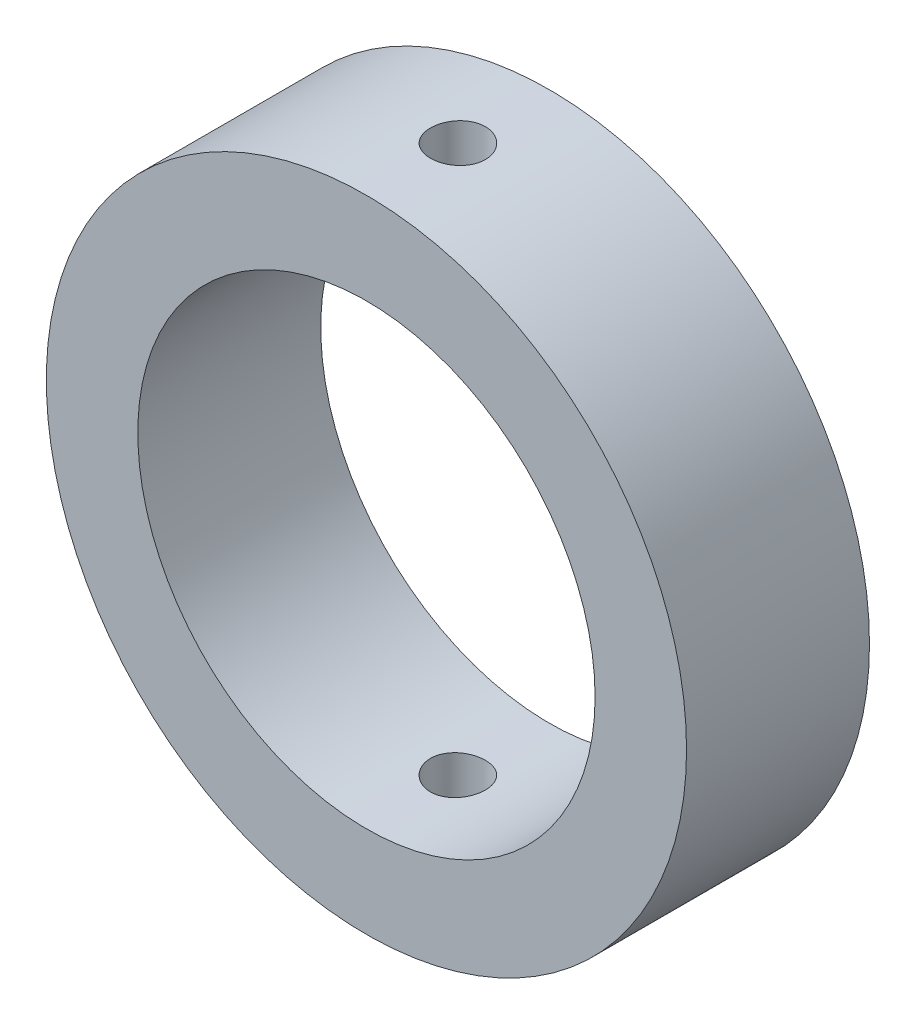
ISO-10303-21;
HEADER;
FILE_DESCRIPTION(('STEP AP214'),'2;1');
FILE_NAME('part.step','',(''),(''),'','','');
FILE_SCHEMA(('AUTOMOTIVE_DESIGN { 1 0 10303 214 1 1 1 1 }'));
ENDSEC;
DATA;
#1=APPLICATION_CONTEXT('core data for automotive mechanical design processes');
#2=APPLICATION_PROTOCOL_DEFINITION('international standard','automotive_design',2000,#1);
#3=PRODUCT_CONTEXT('',#1,'mechanical');
#4=PRODUCT('Part','Part','',(#3));
#5=PRODUCT_RELATED_PRODUCT_CATEGORY('part','',(#4));
#6=PRODUCT_DEFINITION_FORMATION('','',#4);
#7=PRODUCT_DEFINITION_CONTEXT('part definition',#1,'design');
#8=PRODUCT_DEFINITION('design','',#6,#7);
#9=PRODUCT_DEFINITION_SHAPE('','',#8);
#10=(LENGTH_UNIT() NAMED_UNIT(*) SI_UNIT(.MILLI.,.METRE.));
#11=(NAMED_UNIT(*) PLANE_ANGLE_UNIT() SI_UNIT($,.RADIAN.));
#12=(NAMED_UNIT(*) SI_UNIT($,.STERADIAN.) SOLID_ANGLE_UNIT());
#13=UNCERTAINTY_MEASURE_WITH_UNIT(LENGTH_MEASURE(1.E-05),#10,'distance_accuracy_value','');
#14=(GEOMETRIC_REPRESENTATION_CONTEXT(3) GLOBAL_UNCERTAINTY_ASSIGNED_CONTEXT((#13)) GLOBAL_UNIT_ASSIGNED_CONTEXT((#10,
#11,#12)) REPRESENTATION_CONTEXT('',''));
#15=CARTESIAN_POINT('',(0.,0.,0.));
#16=DIRECTION('',(0.,0.,1.));
#17=DIRECTION('',(1.,0.,0.));
#18=AXIS2_PLACEMENT_3D('',#15,#16,#17);
#19=CARTESIAN_POINT('',(0.,0.,20.));
#20=DIRECTION('',(0.,0.,1.));
#21=DIRECTION('',(1.,0.,0.));
#22=AXIS2_PLACEMENT_3D('',#19,#20,#21);
#23=PLANE('',#22);
#24=CARTESIAN_POINT('',(0.,0.,20.));
#25=DIRECTION('',(0.,0.,1.));
#26=DIRECTION('',(1.,0.,0.));
#27=AXIS2_PLACEMENT_3D('',#24,#25,#26);
#28=CIRCLE('',#27,35.);
#29=CARTESIAN_POINT('',(35.,0.,20.));
#30=VERTEX_POINT('',#29);
#31=EDGE_CURVE('E10',#30,#30,#28,.T.);
#32=ORIENTED_EDGE('',*,*,#31,.T.);
#33=EDGE_LOOP('',(#32));
#34=FACE_BOUND('',#33,.T.);
#35=CARTESIAN_POINT('',(0.,0.,20.));
#36=DIRECTION('',(0.,0.,1.));
#37=DIRECTION('',(1.,0.,0.));
#38=AXIS2_PLACEMENT_3D('',#35,#36,#37);
#39=CIRCLE('',#38,25.);
#40=CARTESIAN_POINT('',(25.,0.,20.));
#41=VERTEX_POINT('',#40);
#42=EDGE_CURVE('E57',#41,#41,#39,.T.);
#43=ORIENTED_EDGE('',*,*,#42,.F.);
#44=EDGE_LOOP('',(#43));
#45=FACE_BOUND('',#44,.T.);
#46=ADVANCED_FACE('F40',(#34,#45),#23,.T.);
#47=CARTESIAN_POINT('',(0.,0.,0.));
#48=DIRECTION('',(0.,0.,1.));
#49=DIRECTION('',(1.,0.,0.));
#50=AXIS2_PLACEMENT_3D('',#47,#48,#49);
#51=PLANE('',#50);
#52=CARTESIAN_POINT('',(0.,0.,0.));
#53=DIRECTION('',(0.,0.,1.));
#54=DIRECTION('',(1.,0.,0.));
#55=AXIS2_PLACEMENT_3D('',#52,#53,#54);
#56=CIRCLE('',#55,35.);
#57=CARTESIAN_POINT('',(35.,0.,0.));
#58=VERTEX_POINT('',#57);
#59=EDGE_CURVE('E51',#58,#58,#56,.T.);
#60=ORIENTED_EDGE('',*,*,#59,.F.);
#61=EDGE_LOOP('',(#60));
#62=FACE_BOUND('',#61,.T.);
#63=CARTESIAN_POINT('',(0.,0.,0.));
#64=DIRECTION('',(0.,0.,1.));
#65=DIRECTION('',(1.,0.,0.));
#66=AXIS2_PLACEMENT_3D('',#63,#64,#65);
#67=CIRCLE('',#66,25.);
#68=CARTESIAN_POINT('',(25.,0.,0.));
#69=VERTEX_POINT('',#68);
#70=EDGE_CURVE('E56',#69,#69,#67,.T.);
#71=ORIENTED_EDGE('',*,*,#70,.T.);
#72=EDGE_LOOP('',(#71));
#73=FACE_BOUND('',#72,.T.);
#74=ADVANCED_FACE('F92',(#62,#73),#51,.F.);
#75=CARTESIAN_POINT('',(0.,0.,20.));
#76=DIRECTION('',(0.,0.,-1.));
#77=DIRECTION('',(-1.,0.,0.));
#78=AXIS2_PLACEMENT_3D('',#75,#76,#77);
#79=CYLINDRICAL_SURFACE('',#78,35.);
#80=CARTESIAN_POINT('',(0.,-35.,13.));
#81=CARTESIAN_POINT('',(0.168180177421425,-34.9999983189466,12.9999926621086));
#82=CARTESIAN_POINT('',(0.336474410694065,-34.9987748870089,12.9858101377132));
#83=CARTESIAN_POINT('',(0.668405276387218,-34.9940120055983,12.9294427662291));
#84=CARTESIAN_POINT('',(0.832036433522409,-34.9904699418268,12.8872263096079));
#85=CARTESIAN_POINT('',(1.14978580604665,-34.9814700099417,12.7760219308489));
#86=CARTESIAN_POINT('',(1.30390939390644,-34.9760132356579,12.7070492915307));
#87=CARTESIAN_POINT('',(1.5983553572425,-34.9637955952331,12.5443180840418));
#88=CARTESIAN_POINT('',(1.7386806487592,-34.9570350055299,12.4505647683675));
#89=CARTESIAN_POINT('',(2.00196024172095,-34.9429478698077,12.2406617110507));
#90=CARTESIAN_POINT('',(2.12487233650439,-34.9356200130701,12.1244591132005));
#91=CARTESIAN_POINT('',(2.34947428548936,-34.9212352148941,11.8730679106441));
#92=CARTESIAN_POINT('',(2.45116320107853,-34.9141782854488,11.7378784666713));
#93=CARTESIAN_POINT('',(2.63057608789142,-34.9011203668809,11.4520942390574));
#94=CARTESIAN_POINT('',(2.70826279885841,-34.895121025662,11.3014759820008));
#95=CARTESIAN_POINT('',(2.83722803822898,-34.8848727505605,10.9892731041776));
#96=CARTESIAN_POINT('',(2.88850705745045,-34.8806237841455,10.8276886872931));
#97=CARTESIAN_POINT('',(2.96307845769353,-34.8743684880487,10.4985643557107));
#98=CARTESIAN_POINT('',(2.98643979537529,-34.8723566335604,10.3310401716124));
#99=CARTESIAN_POINT('',(3.00472573441206,-34.8707859372111,9.99443731566983));
#100=CARTESIAN_POINT('',(2.99965089755265,-34.8712270468893,9.82535867460139));
#101=CARTESIAN_POINT('',(2.96126551313284,-34.874507414771,9.49091935009246));
#102=CARTESIAN_POINT('',(2.92802995365881,-34.8773403039272,9.32554998866099));
#103=CARTESIAN_POINT('',(2.83438308452453,-34.8850750500347,9.00274549875546));
#104=CARTESIAN_POINT('',(2.77397149596722,-34.8899769282191,8.84531045172664));
#105=CARTESIAN_POINT('',(2.62760362876988,-34.9013046627491,8.5426048976093));
#106=CARTESIAN_POINT('',(2.54161375570937,-34.9077325210554,8.39735071245931));
#107=CARTESIAN_POINT('',(2.34655446417304,-34.9213861292491,8.12330862382476));
#108=CARTESIAN_POINT('',(2.23748455081154,-34.9286118962437,7.99452107351525));
#109=CARTESIAN_POINT('',(1.99894091774494,-34.9430754969892,7.75663207823613));
#110=CARTESIAN_POINT('',(1.86940237855328,-34.9503132942366,7.64759561833133));
#111=CARTESIAN_POINT('',(1.59382461581758,-34.9639632077666,7.45280656292255));
#112=CARTESIAN_POINT('',(1.44778538038973,-34.9703753234546,7.36705398418779));
#113=CARTESIAN_POINT('',(1.14330913680171,-34.9816527329005,7.2212707481009));
#114=CARTESIAN_POINT('',(0.984870717201058,-34.9865178502383,7.16124302414623));
#115=CARTESIAN_POINT('',(0.66011322112835,-34.9941511080319,7.06865924334512));
#116=CARTESIAN_POINT('',(0.493794317781497,-34.9969192945321,7.03610258328611));
#117=CARTESIAN_POINT('',(0.15856025083397,-35.0000408811527,6.99946669791016));
#118=CARTESIAN_POINT('',(-0.0103450366761302,-35.0004018916599,6.99529772286168));
#119=CARTESIAN_POINT('',(-0.346452104482659,-34.9986887867208,7.01532035576532));
#120=CARTESIAN_POINT('',(-0.513653901587615,-34.9966146953254,7.03951168360929));
#121=CARTESIAN_POINT('',(-0.841351421558966,-34.9902695086844,7.11549382233641));
#122=CARTESIAN_POINT('',(-1.00185687270474,-34.9860017297263,7.16724297716301));
#123=CARTESIAN_POINT('',(-1.31190702245475,-34.9757485102754,7.29682922006561));
#124=CARTESIAN_POINT('',(-1.46145153801856,-34.9697630411066,7.37466674367936));
#125=CARTESIAN_POINT('',(-1.7457428816744,-34.9567262474856,7.55444535294469));
#126=CARTESIAN_POINT('',(-1.88045202960912,-34.9496723123826,7.65644583152676));
#127=CARTESIAN_POINT('',(-2.13086824169311,-34.9352996751561,7.88156921992449));
#128=CARTESIAN_POINT('',(-2.24657495644839,-34.9279809681673,8.00469251803617));
#129=CARTESIAN_POINT('',(-2.45601016602155,-34.9138810732733,8.26895626973909));
#130=CARTESIAN_POINT('',(-2.54968004901865,-34.9071013498897,8.41014326356234));
#131=CARTESIAN_POINT('',(-2.71198063229128,-34.8948680127784,8.70629524502194));
#132=CARTESIAN_POINT('',(-2.78061159495576,-34.8894143851545,8.8612600882557));
#133=CARTESIAN_POINT('',(-2.8907865424564,-34.8804590783594,9.180362211124));
#134=CARTESIAN_POINT('',(-2.93236627395852,-34.8769548240937,9.34448707344406));
#135=CARTESIAN_POINT('',(-2.98737479633476,-34.872286503041,9.67742005737787));
#136=CARTESIAN_POINT('',(-3.0008041627162,-34.871122388412,9.84622808317732));
#137=CARTESIAN_POINT('',(-2.99912392353084,-34.8712668950776,10.1831530647903));
#138=CARTESIAN_POINT('',(-2.98410640669543,-34.8725675374248,10.3512704909289));
#139=CARTESIAN_POINT('',(-2.92615085557176,-34.8774780477604,10.6825859274482));
#140=CARTESIAN_POINT('',(-2.88321277999482,-34.8810879191635,10.8457839305537));
#141=CARTESIAN_POINT('',(-2.7706585792072,-34.8902080316544,11.1626330215739));
#142=CARTESIAN_POINT('',(-2.70104425727074,-34.8957181442861,11.3162847539864));
#143=CARTESIAN_POINT('',(-2.53712384137618,-34.9080181097009,11.6097355757974));
#144=CARTESIAN_POINT('',(-2.4428181018962,-34.9148079441114,11.7495348640265));
#145=CARTESIAN_POINT('',(-2.23184571903132,-34.9289284828144,12.0117838459397));
#146=CARTESIAN_POINT('',(-2.11511080731054,-34.9362607952504,12.1341785330169));
#147=CARTESIAN_POINT('',(-1.86271960746937,-34.9506254222313,12.357688026767));
#148=CARTESIAN_POINT('',(-1.72705875414518,-34.9576576638589,12.4587976843829));
#149=CARTESIAN_POINT('',(-1.44039065385252,-34.9706432183248,12.6370108284413));
#150=CARTESIAN_POINT('',(-1.28935405311577,-34.9765944046818,12.7140672103455));
#151=CARTESIAN_POINT('',(-0.976537475486436,-34.9867226680456,12.8416267776672));
#152=CARTESIAN_POINT('',(-0.814770058056751,-34.9909017781752,12.8921604088507));
#153=CARTESIAN_POINT('',(-0.543377751492647,-34.9959451685553,12.9524054943071));
#154=CARTESIAN_POINT('',(-0.4354969109927,-34.9974587860022,12.9702296244532));
#155=CARTESIAN_POINT('',(-0.218426750644092,-34.999486746251,12.9940292435666));
#156=CARTESIAN_POINT('',(-0.109237434508938,-35.0000010918883,13.0000047661528));
#157=CARTESIAN_POINT('',(0.,-35.,13.));
#158=B_SPLINE_CURVE_WITH_KNOTS('',3,(#80,#81,#82,#83,#84,#85,#86,#87,#88,#89,#90,#91,#92,#93,
#94,#95,#96,#97,#98,#99,#100,#101,#102,#103,#104,#105,#106,#107,#108,#109,#110,#111,#112,#113,
#114,#115,#116,#117,#118,#119,#120,#121,#122,#123,#124,#125,#126,#127,#128,#129,#130,#131,#132,
#133,#134,#135,#136,#137,#138,#139,#140,#141,#142,#143,#144,#145,#146,#147,#148,#149,#150,#151,
#152,#153,#154,#155,#156,#157),.UNSPECIFIED.,.T.,.F.,(4,2,2,2,2,2,2,2,2,2,2,2,2,2,2,2,2,2,2,2,2,
2,2,2,2,2,2,2,2,2,2,2,2,2,2,2,2,2,4),(0.,0.504141688620747,1.00885278730409,1.51327602436422,
2.01759242981481,2.5231110330061,3.0286519884333,3.53497383147415,4.04128626359052,
4.54634550220951,5.05139476290399,5.55510335902216,6.05881712462464,6.56319540924795,
7.06758450992202,7.57360414720597,8.07962414892789,8.58570183661505,9.09176841150507,
9.59623427417642,10.1006951543972,10.6043956535469,11.1081045622491,11.6130646830275,
12.1180340873686,12.6243317573245,13.1306241215114,13.636246082805,14.1418577070399,
14.6458353534655,15.1498137451707,15.6537580747011,16.1576951698375,16.6631911333163,
17.1688092410494,17.6754113983993,18.1814307424438,18.5088849156758,18.8363381597995),.UNSPECIFIED.);
#159=CARTESIAN_POINT('',(0.,-35.,13.));
#160=VERTEX_POINT('',#159);
#161=EDGE_CURVE('E84',#160,#160,#158,.T.);
#162=ORIENTED_EDGE('',*,*,#161,.T.);
#163=EDGE_LOOP('',(#162));
#164=FACE_BOUND('',#163,.T.);
#165=CARTESIAN_POINT('',(0.,35.,13.));
#166=CARTESIAN_POINT('',(-0.168180177421425,34.9999983189466,12.9999926621086));
#167=CARTESIAN_POINT('',(-0.336474410694065,34.9987748870089,12.9858101377132));
#168=CARTESIAN_POINT('',(-0.668405276387218,34.9940120055983,12.9294427662291));
#169=CARTESIAN_POINT('',(-0.832036433522409,34.9904699418268,12.8872263096079));
#170=CARTESIAN_POINT('',(-1.14978580604665,34.9814700099417,12.7760219308489));
#171=CARTESIAN_POINT('',(-1.30390939390644,34.9760132356579,12.7070492915307));
#172=CARTESIAN_POINT('',(-1.5983553572425,34.9637955952331,12.5443180840418));
#173=CARTESIAN_POINT('',(-1.7386806487592,34.9570350055299,12.4505647683675));
#174=CARTESIAN_POINT('',(-2.00196024172095,34.9429478698077,12.2406617110507));
#175=CARTESIAN_POINT('',(-2.12487233650439,34.9356200130701,12.1244591132005));
#176=CARTESIAN_POINT('',(-2.34947428548936,34.9212352148941,11.8730679106441));
#177=CARTESIAN_POINT('',(-2.45116320107853,34.9141782854488,11.7378784666713));
#178=CARTESIAN_POINT('',(-2.63057608789142,34.9011203668809,11.4520942390574));
#179=CARTESIAN_POINT('',(-2.70826279885841,34.895121025662,11.3014759820008));
#180=CARTESIAN_POINT('',(-2.83722803822898,34.8848727505605,10.9892731041776));
#181=CARTESIAN_POINT('',(-2.88850705745045,34.8806237841455,10.8276886872931));
#182=CARTESIAN_POINT('',(-2.96307845769353,34.8743684880487,10.4985643557107));
#183=CARTESIAN_POINT('',(-2.98643979537529,34.8723566335604,10.3310401716124));
#184=CARTESIAN_POINT('',(-3.00472573441206,34.8707859372111,9.99443731566983));
#185=CARTESIAN_POINT('',(-2.99965089755265,34.8712270468893,9.82535867460139));
#186=CARTESIAN_POINT('',(-2.96126551313284,34.874507414771,9.49091935009246));
#187=CARTESIAN_POINT('',(-2.92802995365881,34.8773403039272,9.32554998866099));
#188=CARTESIAN_POINT('',(-2.83438308452453,34.8850750500347,9.00274549875546));
#189=CARTESIAN_POINT('',(-2.77397149596722,34.8899769282191,8.84531045172664));
#190=CARTESIAN_POINT('',(-2.62760362876988,34.9013046627491,8.5426048976093));
#191=CARTESIAN_POINT('',(-2.54161375570937,34.9077325210554,8.39735071245931));
#192=CARTESIAN_POINT('',(-2.34655446417304,34.9213861292491,8.12330862382476));
#193=CARTESIAN_POINT('',(-2.23748455081154,34.9286118962437,7.99452107351525));
#194=CARTESIAN_POINT('',(-1.99894091774494,34.9430754969892,7.75663207823613));
#195=CARTESIAN_POINT('',(-1.86940237855328,34.9503132942366,7.64759561833133));
#196=CARTESIAN_POINT('',(-1.59382461581758,34.9639632077666,7.45280656292255));
#197=CARTESIAN_POINT('',(-1.44778538038973,34.9703753234546,7.36705398418779));
#198=CARTESIAN_POINT('',(-1.14330913680171,34.9816527329005,7.2212707481009));
#199=CARTESIAN_POINT('',(-0.984870717201058,34.9865178502383,7.16124302414623));
#200=CARTESIAN_POINT('',(-0.66011322112835,34.9941511080319,7.06865924334512));
#201=CARTESIAN_POINT('',(-0.493794317781497,34.9969192945321,7.03610258328611));
#202=CARTESIAN_POINT('',(-0.15856025083397,35.0000408811527,6.99946669791016));
#203=CARTESIAN_POINT('',(0.0103450366761302,35.0004018916599,6.99529772286168));
#204=CARTESIAN_POINT('',(0.346452104482659,34.9986887867208,7.01532035576532));
#205=CARTESIAN_POINT('',(0.513653901587615,34.9966146953254,7.03951168360929));
#206=CARTESIAN_POINT('',(0.841351421558966,34.9902695086844,7.11549382233641));
#207=CARTESIAN_POINT('',(1.00185687270474,34.9860017297263,7.16724297716301));
#208=CARTESIAN_POINT('',(1.31190702245475,34.9757485102754,7.29682922006561));
#209=CARTESIAN_POINT('',(1.46145153801856,34.9697630411066,7.37466674367936));
#210=CARTESIAN_POINT('',(1.7457428816744,34.9567262474856,7.55444535294469));
#211=CARTESIAN_POINT('',(1.88045202960912,34.9496723123826,7.65644583152676));
#212=CARTESIAN_POINT('',(2.13086824169311,34.9352996751561,7.88156921992449));
#213=CARTESIAN_POINT('',(2.24657495644839,34.9279809681673,8.00469251803617));
#214=CARTESIAN_POINT('',(2.45601016602155,34.9138810732733,8.26895626973909));
#215=CARTESIAN_POINT('',(2.54968004901865,34.9071013498897,8.41014326356234));
#216=CARTESIAN_POINT('',(2.71198063229128,34.8948680127784,8.70629524502194));
#217=CARTESIAN_POINT('',(2.78061159495576,34.8894143851545,8.8612600882557));
#218=CARTESIAN_POINT('',(2.8907865424564,34.8804590783594,9.180362211124));
#219=CARTESIAN_POINT('',(2.93236627395852,34.8769548240937,9.34448707344406));
#220=CARTESIAN_POINT('',(2.98737479633476,34.872286503041,9.67742005737787));
#221=CARTESIAN_POINT('',(3.0008041627162,34.871122388412,9.84622808317732));
#222=CARTESIAN_POINT('',(2.99912392353084,34.8712668950776,10.1831530647903));
#223=CARTESIAN_POINT('',(2.98410640669543,34.8725675374248,10.3512704909289));
#224=CARTESIAN_POINT('',(2.92615085557176,34.8774780477604,10.6825859274482));
#225=CARTESIAN_POINT('',(2.88321277999482,34.8810879191635,10.8457839305537));
#226=CARTESIAN_POINT('',(2.7706585792072,34.8902080316544,11.1626330215739));
#227=CARTESIAN_POINT('',(2.70104425727074,34.8957181442861,11.3162847539864));
#228=CARTESIAN_POINT('',(2.53712384137618,34.9080181097009,11.6097355757974));
#229=CARTESIAN_POINT('',(2.4428181018962,34.9148079441114,11.7495348640265));
#230=CARTESIAN_POINT('',(2.23184571903132,34.9289284828144,12.0117838459397));
#231=CARTESIAN_POINT('',(2.11511080731054,34.9362607952504,12.1341785330169));
#232=CARTESIAN_POINT('',(1.86271960746937,34.9506254222313,12.357688026767));
#233=CARTESIAN_POINT('',(1.72705875414518,34.9576576638589,12.4587976843829));
#234=CARTESIAN_POINT('',(1.44039065385252,34.9706432183248,12.6370108284413));
#235=CARTESIAN_POINT('',(1.28935405311577,34.9765944046818,12.7140672103455));
#236=CARTESIAN_POINT('',(0.976537475486436,34.9867226680456,12.8416267776672));
#237=CARTESIAN_POINT('',(0.814770058056751,34.9909017781752,12.8921604088507));
#238=CARTESIAN_POINT('',(0.543377751492647,34.9959451685553,12.9524054943071));
#239=CARTESIAN_POINT('',(0.4354969109927,34.9974587860022,12.9702296244532));
#240=CARTESIAN_POINT('',(0.218426750644092,34.999486746251,12.9940292435666));
#241=CARTESIAN_POINT('',(0.109237434508938,35.0000010918883,13.0000047661528));
#242=CARTESIAN_POINT('',(0.,35.,13.));
#243=B_SPLINE_CURVE_WITH_KNOTS('',3,(#165,#166,#167,#168,#169,#170,#171,#172,#173,#174,#175,
#176,#177,#178,#179,#180,#181,#182,#183,#184,#185,#186,#187,#188,#189,#190,#191,#192,#193,#194,
#195,#196,#197,#198,#199,#200,#201,#202,#203,#204,#205,#206,#207,#208,#209,#210,#211,#212,#213,
#214,#215,#216,#217,#218,#219,#220,#221,#222,#223,#224,#225,#226,#227,#228,#229,#230,#231,#232,
#233,#234,#235,#236,#237,#238,#239,#240,#241,#242),.UNSPECIFIED.,.T.,.F.,(4,2,2,2,2,2,2,2,2,2,2,
2,2,2,2,2,2,2,2,2,2,2,2,2,2,2,2,2,2,2,2,2,2,2,2,2,2,2,4),(0.,0.504141688620747,1.00885278730409,
1.51327602436422,2.01759242981481,2.5231110330061,3.0286519884333,3.53497383147415,
4.04128626359052,4.54634550220951,5.05139476290399,5.55510335902216,6.05881712462464,
6.56319540924795,7.06758450992202,7.57360414720597,8.07962414892789,8.58570183661505,
9.09176841150507,9.59623427417642,10.1006951543972,10.6043956535469,11.1081045622491,
11.6130646830275,12.1180340873686,12.6243317573245,13.1306241215114,13.636246082805,
14.1418577070399,14.6458353534655,15.1498137451707,15.6537580747011,16.1576951698375,
16.6631911333163,17.1688092410494,17.6754113983993,18.1814307424438,18.5088849156758,
18.8363381597995),.UNSPECIFIED.);
#244=CARTESIAN_POINT('',(0.,35.,13.));
#245=VERTEX_POINT('',#244);
#246=EDGE_CURVE('E76',#245,#245,#243,.T.);
#247=ORIENTED_EDGE('',*,*,#246,.T.);
#248=EDGE_LOOP('',(#247));
#249=FACE_BOUND('',#248,.T.);
#250=ORIENTED_EDGE('',*,*,#31,.F.);
#251=EDGE_LOOP('',(#250));
#252=FACE_BOUND('',#251,.T.);
#253=ORIENTED_EDGE('',*,*,#59,.T.);
#254=EDGE_LOOP('',(#253));
#255=FACE_BOUND('',#254,.T.);
#256=ADVANCED_FACE('F39',(#164,#249,#252,#255),#79,.T.);
#257=CARTESIAN_POINT('',(0.,0.,20.));
#258=DIRECTION('',(0.,0.,-1.));
#259=DIRECTION('',(-1.,0.,0.));
#260=AXIS2_PLACEMENT_3D('',#257,#258,#259);
#261=CYLINDRICAL_SURFACE('',#260,25.);
#262=CARTESIAN_POINT('',(0.,-25.,13.));
#263=CARTESIAN_POINT('',(0.167864047107699,-24.9999977357459,12.9999928360586));
#264=CARTESIAN_POINT('',(0.335834317331191,-24.9982914200408,12.9858633413073));
#265=CARTESIAN_POINT('',(0.66710457130825,-24.991648705422,12.9297189358446));
#266=CARTESIAN_POINT('',(0.830399429590069,-24.9867088933728,12.8876745587494));
#267=CARTESIAN_POINT('',(1.14747479534053,-24.9741559265426,12.776953723474));
#268=CARTESIAN_POINT('',(1.30126148759225,-24.9665445315309,12.7082947931758));
#269=CARTESIAN_POINT('',(1.595099157832,-24.9494959264345,12.5463312649167));
#270=CARTESIAN_POINT('',(1.73515256713516,-24.9400590404141,12.4530310402467));
#271=CARTESIAN_POINT('',(1.99829131534451,-24.920360105442,12.2439251380248));
#272=CARTESIAN_POINT('',(2.1212966913072,-24.9100945030904,12.1280191598881));
#273=CARTESIAN_POINT('',(2.34615931038342,-24.8899239397152,11.8772070351121));
#274=CARTESIAN_POINT('',(2.44801549826474,-24.8800189967068,11.7422999409814));
#275=CARTESIAN_POINT('',(2.62798342873896,-24.8616560370405,11.4567991747016));
#276=CARTESIAN_POINT('',(2.7060207567257,-24.8532025903971,11.3061582754199));
#277=CARTESIAN_POINT('',(2.8356605730156,-24.8387461344686,10.9937912978913));
#278=CARTESIAN_POINT('',(2.88726398696776,-24.8327430393798,10.8320656080307));
#279=CARTESIAN_POINT('',(2.96232930045399,-24.8239006073737,10.5029471406886));
#280=CARTESIAN_POINT('',(2.98592577987646,-24.8210461452543,10.3355854715723));
#281=CARTESIAN_POINT('',(3.0047237521967,-24.8187777690611,9.99925506363583));
#282=CARTESIAN_POINT('',(2.99992630052848,-24.8193637271033,9.83028638478303));
#283=CARTESIAN_POINT('',(2.96218316078668,-24.8238961466306,9.49647403521565));
#284=CARTESIAN_POINT('',(2.92938543222303,-24.8278249434675,9.33161336131982));
#285=CARTESIAN_POINT('',(2.83680346170067,-24.8385728087608,9.00975297217864));
#286=CARTESIAN_POINT('',(2.77701871225814,-24.8453919315688,8.85275340482101));
#287=CARTESIAN_POINT('',(2.63199980699862,-24.8611722079476,8.55061053176089));
#288=CARTESIAN_POINT('',(2.54670106203925,-24.8701387862198,8.40549852164644));
#289=CARTESIAN_POINT('',(2.35312173169469,-24.8891993987901,8.13159278908424));
#290=CARTESIAN_POINT('',(2.24484017723157,-24.8992934806213,8.00279975509743));
#291=CARTESIAN_POINT('',(2.0075475556218,-24.9195503308637,7.76432891563562));
#292=CARTESIAN_POINT('',(1.87840890051216,-24.929713127424,7.65477803014294));
#293=CARTESIAN_POINT('',(1.60350795893872,-24.9489020798549,7.45888847899969));
#294=CARTESIAN_POINT('',(1.45774563908005,-24.9579282334421,7.37254985998085));
#295=CARTESIAN_POINT('',(1.15363930826285,-24.9738318861702,7.22553671436034));
#296=CARTESIAN_POINT('',(0.995291578715591,-24.9807087472809,7.16486980666956));
#297=CARTESIAN_POINT('',(0.67055602227344,-24.991533065309,7.0710212621491));
#298=CARTESIAN_POINT('',(0.504168542441623,-24.9954806485584,7.03783843999552));
#299=CARTESIAN_POINT('',(0.169174396374217,-24.9999852500304,7.00006374450231));
#300=CARTESIAN_POINT('',(0.000587720432051526,-25.0005630093753,6.9952969675993));
#301=CARTESIAN_POINT('',(-0.33498206824326,-24.9983187823231,7.01402857786827));
#302=CARTESIAN_POINT('',(-0.501965212327328,-24.9954968625308,7.03752641129535));
#303=CARTESIAN_POINT('',(-0.829074263928356,-24.9867833380686,7.11197496400309));
#304=CARTESIAN_POINT('',(-0.989219346369035,-24.9809010237909,7.16284261305008));
#305=CARTESIAN_POINT('',(-1.29870539768646,-24.9667255501792,7.29050070335358));
#306=CARTESIAN_POINT('',(-1.44804602592347,-24.9584323148759,7.36729196149009));
#307=CARTESIAN_POINT('',(-1.73246717766504,-24.9403085158695,7.54504291590243));
#308=CARTESIAN_POINT('',(-1.86747628962751,-24.9304708084643,7.64611613781082));
#309=CARTESIAN_POINT('',(-2.11867625152203,-24.9103817919419,7.86940084640817));
#310=CARTESIAN_POINT('',(-2.23486641472949,-24.9001304677484,7.99161310414795));
#311=CARTESIAN_POINT('',(-2.44574795226154,-24.8803059484942,8.25447561542769));
#312=CARTESIAN_POINT('',(-2.54032363231939,-24.8707365831307,8.39521901534385));
#313=CARTESIAN_POINT('',(-2.70449314429332,-24.8534214993383,8.69069502507556));
#314=CARTESIAN_POINT('',(-2.77408744356074,-24.8456757467943,8.84542737311824));
#315=CARTESIAN_POINT('',(-2.88612996668159,-24.8329105734502,9.1641106088947));
#316=CARTESIAN_POINT('',(-2.92864420159346,-24.8278845275633,9.32803801185939));
#317=CARTESIAN_POINT('',(-2.98553272163516,-24.8211085274587,9.66076896948507));
#318=CARTESIAN_POINT('',(-2.99990820526081,-24.8193584337106,9.82957231615732));
#319=CARTESIAN_POINT('',(-3.00009033817931,-24.819336326607,10.1661127296372));
#320=CARTESIAN_POINT('',(-2.98607873671351,-24.8210421863943,10.3338497257713));
#321=CARTESIAN_POINT('',(-2.93026848672089,-24.8276922947425,10.6645667863942));
#322=CARTESIAN_POINT('',(-2.88846982822067,-24.8326365444656,10.8275468491756));
#323=CARTESIAN_POINT('',(-2.77832739820545,-24.8451996524586,11.1441045388887));
#324=CARTESIAN_POINT('',(-2.70999165570539,-24.8528177016812,11.2976849934955));
#325=CARTESIAN_POINT('',(-2.5487328262801,-24.8698714539139,11.5912277470701));
#326=CARTESIAN_POINT('',(-2.45580952709445,-24.8793071726153,11.7311899284593));
#327=CARTESIAN_POINT('',(-2.24733689647205,-24.8990055122588,11.9944529401088));
#328=CARTESIAN_POINT('',(-2.1316520393015,-24.9092728581347,12.1176461032663));
#329=CARTESIAN_POINT('',(-1.88122093334447,-24.9294354968169,12.342942479566));
#330=CARTESIAN_POINT('',(-1.74647018263601,-24.939330701051,12.4450406976292));
#331=CARTESIAN_POINT('',(-1.46119322465137,-24.9576721709324,12.6255505779989));
#332=CARTESIAN_POINT('',(-1.31061323462417,-24.966113221621,12.7038777257223));
#333=CARTESIAN_POINT('',(-0.99842275168531,-24.9805418519727,12.8340237644426));
#334=CARTESIAN_POINT('',(-0.836824564362144,-24.9865321180615,12.8858716961804));
#335=CARTESIAN_POINT('',(-0.561977101236697,-24.9939268325999,12.9490634203381));
#336=CARTESIAN_POINT('',(-0.450466569753487,-24.996193279433,12.9681374838864));
#337=CARTESIAN_POINT('',(-0.225986735693694,-24.9992306204204,12.993608143491));
#338=CARTESIAN_POINT('',(-0.113017442753625,-25.0000015244492,13.0000048232505));
#339=CARTESIAN_POINT('',(0.,-25.,13.));
#340=B_SPLINE_CURVE_WITH_KNOTS('',3,(#262,#263,#264,#265,#266,#267,#268,#269,#270,#271,#272,
#273,#274,#275,#276,#277,#278,#279,#280,#281,#282,#283,#284,#285,#286,#287,#288,#289,#290,#291,
#292,#293,#294,#295,#296,#297,#298,#299,#300,#301,#302,#303,#304,#305,#306,#307,#308,#309,#310,
#311,#312,#313,#314,#315,#316,#317,#318,#319,#320,#321,#322,#323,#324,#325,#326,#327,#328,#329,
#330,#331,#332,#333,#334,#335,#336,#337,#338,#339),.UNSPECIFIED.,.T.,.F.,(4,2,2,2,2,2,2,2,2,2,2,
2,2,2,2,2,2,2,2,2,2,2,2,2,2,2,2,2,2,2,2,2,2,2,2,2,2,2,4),(0.,0.503179350956159,1.00689069408623,
1.5102708637556,2.01356175441693,2.51913872195878,3.02474090904883,3.53190689496397,
4.03905511999113,4.54375638343279,5.0484388866848,5.55047092912253,6.05251241253396,
6.55583573710536,7.05918028869262,7.56572944640317,8.07227962172601,8.57898002694278,
9.08565857822619,9.58921522624226,10.0927620090108,10.5947890255775,11.0968318630167,
11.6012692178556,12.1057249760356,12.6128207581672,13.119907053063,13.6257524826489,
14.1315763666154,14.6341719319229,15.1367676776234,15.6392114771388,16.1416596143122,
16.6471952402032,17.1528504352009,17.6602829023946,18.1671576479275,18.5059342945627,
18.8447087043981),.UNSPECIFIED.);
#341=CARTESIAN_POINT('',(0.,-25.,13.));
#342=VERTEX_POINT('',#341);
#343=EDGE_CURVE('E45',#342,#342,#340,.T.);
#344=ORIENTED_EDGE('',*,*,#343,.F.);
#345=EDGE_LOOP('',(#344));
#346=FACE_BOUND('',#345,.T.);
#347=CARTESIAN_POINT('',(0.,25.,13.));
#348=CARTESIAN_POINT('',(-0.167864047107699,24.9999977357459,12.9999928360586));
#349=CARTESIAN_POINT('',(-0.335834317331191,24.9982914200408,12.9858633413073));
#350=CARTESIAN_POINT('',(-0.66710457130825,24.991648705422,12.9297189358446));
#351=CARTESIAN_POINT('',(-0.830399429590069,24.9867088933728,12.8876745587494));
#352=CARTESIAN_POINT('',(-1.14747479534053,24.9741559265426,12.776953723474));
#353=CARTESIAN_POINT('',(-1.30126148759225,24.9665445315309,12.7082947931758));
#354=CARTESIAN_POINT('',(-1.595099157832,24.9494959264345,12.5463312649167));
#355=CARTESIAN_POINT('',(-1.73515256713516,24.9400590404141,12.4530310402467));
#356=CARTESIAN_POINT('',(-1.99829131534451,24.920360105442,12.2439251380248));
#357=CARTESIAN_POINT('',(-2.1212966913072,24.9100945030904,12.1280191598881));
#358=CARTESIAN_POINT('',(-2.34615931038342,24.8899239397152,11.8772070351121));
#359=CARTESIAN_POINT('',(-2.44801549826474,24.8800189967068,11.7422999409814));
#360=CARTESIAN_POINT('',(-2.62798342873896,24.8616560370405,11.4567991747016));
#361=CARTESIAN_POINT('',(-2.7060207567257,24.8532025903971,11.3061582754199));
#362=CARTESIAN_POINT('',(-2.8356605730156,24.8387461344686,10.9937912978913));
#363=CARTESIAN_POINT('',(-2.88726398696776,24.8327430393798,10.8320656080307));
#364=CARTESIAN_POINT('',(-2.96232930045399,24.8239006073737,10.5029471406886));
#365=CARTESIAN_POINT('',(-2.98592577987646,24.8210461452543,10.3355854715723));
#366=CARTESIAN_POINT('',(-3.0047237521967,24.8187777690611,9.99925506363583));
#367=CARTESIAN_POINT('',(-2.99992630052848,24.8193637271033,9.83028638478303));
#368=CARTESIAN_POINT('',(-2.96218316078668,24.8238961466306,9.49647403521565));
#369=CARTESIAN_POINT('',(-2.92938543222303,24.8278249434675,9.33161336131982));
#370=CARTESIAN_POINT('',(-2.83680346170067,24.8385728087608,9.00975297217864));
#371=CARTESIAN_POINT('',(-2.77701871225814,24.8453919315688,8.85275340482101));
#372=CARTESIAN_POINT('',(-2.63199980699862,24.8611722079476,8.55061053176089));
#373=CARTESIAN_POINT('',(-2.54670106203925,24.8701387862198,8.40549852164644));
#374=CARTESIAN_POINT('',(-2.35312173169469,24.8891993987901,8.13159278908424));
#375=CARTESIAN_POINT('',(-2.24484017723157,24.8992934806213,8.00279975509743));
#376=CARTESIAN_POINT('',(-2.0075475556218,24.9195503308637,7.76432891563562));
#377=CARTESIAN_POINT('',(-1.87840890051216,24.929713127424,7.65477803014294));
#378=CARTESIAN_POINT('',(-1.60350795893872,24.9489020798549,7.45888847899969));
#379=CARTESIAN_POINT('',(-1.45774563908005,24.9579282334421,7.37254985998085));
#380=CARTESIAN_POINT('',(-1.15363930826285,24.9738318861702,7.22553671436034));
#381=CARTESIAN_POINT('',(-0.995291578715591,24.9807087472809,7.16486980666956));
#382=CARTESIAN_POINT('',(-0.67055602227344,24.991533065309,7.0710212621491));
#383=CARTESIAN_POINT('',(-0.504168542441623,24.9954806485584,7.03783843999552));
#384=CARTESIAN_POINT('',(-0.169174396374217,24.9999852500304,7.00006374450231));
#385=CARTESIAN_POINT('',(-0.000587720432051526,25.0005630093753,6.9952969675993));
#386=CARTESIAN_POINT('',(0.33498206824326,24.9983187823231,7.01402857786827));
#387=CARTESIAN_POINT('',(0.501965212327328,24.9954968625308,7.03752641129535));
#388=CARTESIAN_POINT('',(0.829074263928356,24.9867833380686,7.11197496400309));
#389=CARTESIAN_POINT('',(0.989219346369035,24.9809010237909,7.16284261305008));
#390=CARTESIAN_POINT('',(1.29870539768646,24.9667255501792,7.29050070335358));
#391=CARTESIAN_POINT('',(1.44804602592347,24.9584323148759,7.36729196149009));
#392=CARTESIAN_POINT('',(1.73246717766504,24.9403085158695,7.54504291590243));
#393=CARTESIAN_POINT('',(1.86747628962751,24.9304708084643,7.64611613781082));
#394=CARTESIAN_POINT('',(2.11867625152203,24.9103817919419,7.86940084640817));
#395=CARTESIAN_POINT('',(2.23486641472949,24.9001304677484,7.99161310414795));
#396=CARTESIAN_POINT('',(2.44574795226154,24.8803059484942,8.25447561542769));
#397=CARTESIAN_POINT('',(2.54032363231939,24.8707365831307,8.39521901534385));
#398=CARTESIAN_POINT('',(2.70449314429332,24.8534214993383,8.69069502507556));
#399=CARTESIAN_POINT('',(2.77408744356074,24.8456757467943,8.84542737311824));
#400=CARTESIAN_POINT('',(2.88612996668159,24.8329105734502,9.1641106088947));
#401=CARTESIAN_POINT('',(2.92864420159346,24.8278845275633,9.32803801185939));
#402=CARTESIAN_POINT('',(2.98553272163516,24.8211085274587,9.66076896948507));
#403=CARTESIAN_POINT('',(2.99990820526081,24.8193584337106,9.82957231615732));
#404=CARTESIAN_POINT('',(3.00009033817931,24.819336326607,10.1661127296372));
#405=CARTESIAN_POINT('',(2.98607873671351,24.8210421863943,10.3338497257713));
#406=CARTESIAN_POINT('',(2.93026848672089,24.8276922947425,10.6645667863942));
#407=CARTESIAN_POINT('',(2.88846982822067,24.8326365444656,10.8275468491756));
#408=CARTESIAN_POINT('',(2.77832739820545,24.8451996524586,11.1441045388887));
#409=CARTESIAN_POINT('',(2.70999165570539,24.8528177016812,11.2976849934955));
#410=CARTESIAN_POINT('',(2.5487328262801,24.8698714539139,11.5912277470701));
#411=CARTESIAN_POINT('',(2.45580952709445,24.8793071726153,11.7311899284593));
#412=CARTESIAN_POINT('',(2.24733689647205,24.8990055122588,11.9944529401088));
#413=CARTESIAN_POINT('',(2.1316520393015,24.9092728581347,12.1176461032663));
#414=CARTESIAN_POINT('',(1.88122093334447,24.9294354968169,12.342942479566));
#415=CARTESIAN_POINT('',(1.74647018263601,24.939330701051,12.4450406976292));
#416=CARTESIAN_POINT('',(1.46119322465137,24.9576721709324,12.6255505779989));
#417=CARTESIAN_POINT('',(1.31061323462417,24.966113221621,12.7038777257223));
#418=CARTESIAN_POINT('',(0.99842275168531,24.9805418519727,12.8340237644426));
#419=CARTESIAN_POINT('',(0.836824564362144,24.9865321180615,12.8858716961804));
#420=CARTESIAN_POINT('',(0.561977101236697,24.9939268325999,12.9490634203381));
#421=CARTESIAN_POINT('',(0.450466569753487,24.996193279433,12.9681374838864));
#422=CARTESIAN_POINT('',(0.225986735693694,24.9992306204204,12.993608143491));
#423=CARTESIAN_POINT('',(0.113017442753625,25.0000015244492,13.0000048232505));
#424=CARTESIAN_POINT('',(0.,25.,13.));
#425=B_SPLINE_CURVE_WITH_KNOTS('',3,(#347,#348,#349,#350,#351,#352,#353,#354,#355,#356,#357,
#358,#359,#360,#361,#362,#363,#364,#365,#366,#367,#368,#369,#370,#371,#372,#373,#374,#375,#376,
#377,#378,#379,#380,#381,#382,#383,#384,#385,#386,#387,#388,#389,#390,#391,#392,#393,#394,#395,
#396,#397,#398,#399,#400,#401,#402,#403,#404,#405,#406,#407,#408,#409,#410,#411,#412,#413,#414,
#415,#416,#417,#418,#419,#420,#421,#422,#423,#424),.UNSPECIFIED.,.T.,.F.,(4,2,2,2,2,2,2,2,2,2,2,
2,2,2,2,2,2,2,2,2,2,2,2,2,2,2,2,2,2,2,2,2,2,2,2,2,2,2,4),(0.,0.503179350956159,1.00689069408623,
1.5102708637556,2.01356175441693,2.51913872195878,3.02474090904883,3.53190689496397,
4.03905511999113,4.54375638343279,5.0484388866848,5.55047092912253,6.05251241253396,
6.55583573710536,7.05918028869262,7.56572944640317,8.07227962172601,8.57898002694278,
9.08565857822619,9.58921522624226,10.0927620090108,10.5947890255775,11.0968318630167,
11.6012692178556,12.1057249760356,12.6128207581672,13.119907053063,13.6257524826489,
14.1315763666154,14.6341719319229,15.1367676776234,15.6392114771388,16.1416596143122,
16.6471952402032,17.1528504352009,17.6602829023946,18.1671576479275,18.5059342945627,
18.8447087043981),.UNSPECIFIED.);
#426=CARTESIAN_POINT('',(0.,25.,13.));
#427=VERTEX_POINT('',#426);
#428=EDGE_CURVE('E62',#427,#427,#425,.T.);
#429=ORIENTED_EDGE('',*,*,#428,.F.);
#430=EDGE_LOOP('',(#429));
#431=FACE_BOUND('',#430,.T.);
#432=ORIENTED_EDGE('',*,*,#42,.T.);
#433=EDGE_LOOP('',(#432));
#434=FACE_BOUND('',#433,.T.);
#435=ORIENTED_EDGE('',*,*,#70,.F.);
#436=EDGE_LOOP('',(#435));
#437=FACE_BOUND('',#436,.T.);
#438=ADVANCED_FACE('F67',(#346,#431,#434,#437),#261,.F.);
#439=CARTESIAN_POINT('',(0.,-35.,10.));
#440=DIRECTION('',(0.,1.,0.));
#441=DIRECTION('',(0.,0.,1.));
#442=AXIS2_PLACEMENT_3D('',#439,#440,#441);
#443=CYLINDRICAL_SURFACE('',#442,3.);
#444=ORIENTED_EDGE('',*,*,#428,.T.);
#445=EDGE_LOOP('',(#444));
#446=FACE_BOUND('',#445,.T.);
#447=ORIENTED_EDGE('',*,*,#246,.F.);
#448=EDGE_LOOP('',(#447));
#449=FACE_BOUND('',#448,.T.);
#450=ADVANCED_FACE('F75',(#446,#449),#443,.F.);
#451=ORIENTED_EDGE('',*,*,#343,.T.);
#452=EDGE_LOOP('',(#451));
#453=FACE_BOUND('',#452,.T.);
#454=ORIENTED_EDGE('',*,*,#161,.F.);
#455=EDGE_LOOP('',(#454));
#456=FACE_BOUND('',#455,.T.);
#457=ADVANCED_FACE('F69',(#453,#456),#443,.F.);
#458=CLOSED_SHELL('',(#46,#74,#256,#438,#450,#457));
#459=MANIFOLD_SOLID_BREP('B2',#458);
#460=ADVANCED_BREP_SHAPE_REPRESENTATION('',(#18,#459),#14);
#461=SHAPE_DEFINITION_REPRESENTATION(#9,#460);
ENDSEC;
END-ISO-10303-21;
